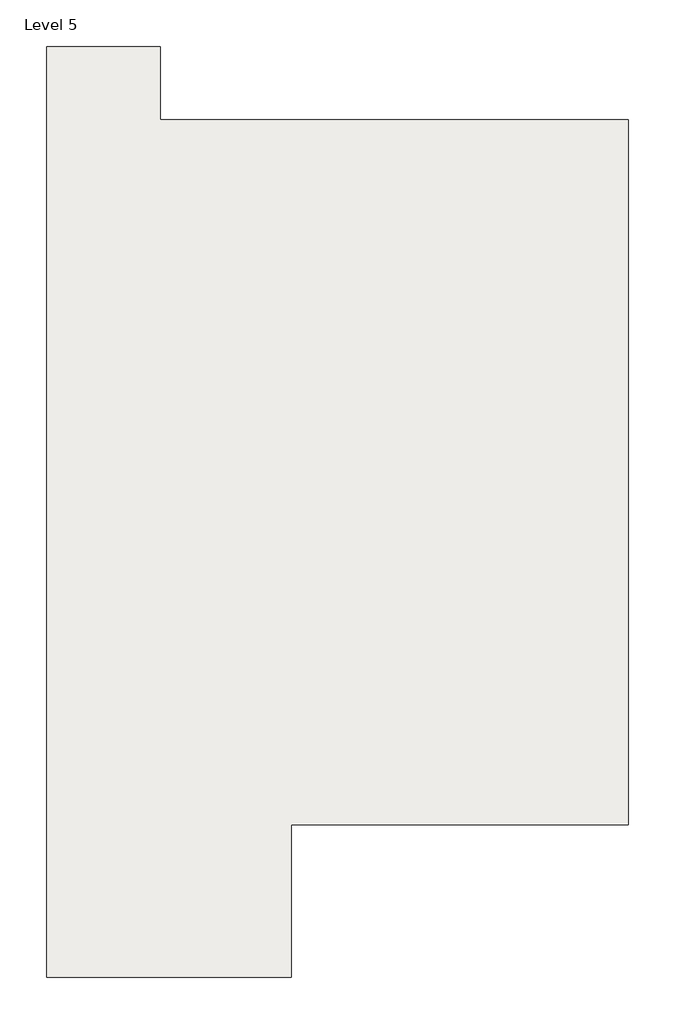
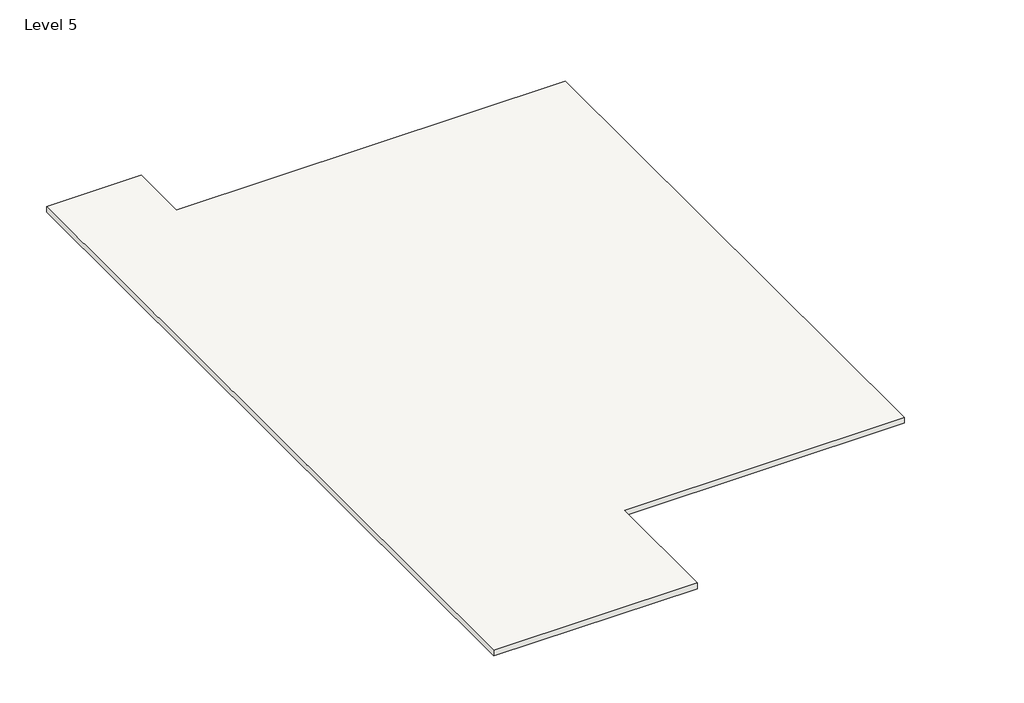
# One storey: 1 roof.
"""IFC4 building model written with IfcOpenShell, lengths in millimetres."""

from ifc_helpers import new_model, si_unit, frame, origin, place, context, project, spatial, polyline, outline, extrude, element, save

model = new_model("IFC4")

# Units and contexts
model_context = context("Model", 3, world=origin())
ifc_project = project(units=[si_unit("LENGTHUNIT", "METRE", prefix="MILLI")], contexts=[model_context])

# Site, building, storey
site = spatial("IfcSite", under=ifc_project)
building = spatial("IfcBuilding", under=site)
storey = spatial("IfcBuildingStorey", under=building, Name="Level 5", Elevation=8077.2)

# Roof
placement = place(None, origin())
element("IfcRoof", 1, ObjectType="6\" roof", at=placement, inside=storey, context=model_context, shape_type="SweptSolid", body=[
    extrude(outline(polyline([(-5248.2909398, -5974.2380415), (-10544.1909398, -5974.2380415), (-10544.1909398, 14151.9493277), (-8080.9689749, 14151.9493277), (-8080.9689749, 12570.5351975), (2028.8090602, 12570.5351975), (2028.8090602, -2669.4648025), (-5248.2909398, -2669.4648025), (-5248.2909398, -5974.2380415)])), frame((0.0, 0.0, 8077.2), z_axis=(0.0, 0.0, 1.0), x_axis=(1.0, 0.0, 0.0)), (0.0, 0.0, 1.0), 152.4),
])

save(model, "model.ifc")

# Revit data of these elements
# Type "6\" roof"
#   Assembly Code = "B1020"
#   Layers, outside or top first: 0' - 6" no material (function 1)
# Element 1 (IfcRoof, "6\" roof")
#   built-in parameter 1001705 = 27 (stored number, unit not read)
#   built-in parameter 1001710 = 33615
#   Phase Created = New Construction
#   Materials on its faces: "Default Roof"
# Materials
#   "Default Roof": colour RGB 88 101 114, transparency 0, Cost = 0
